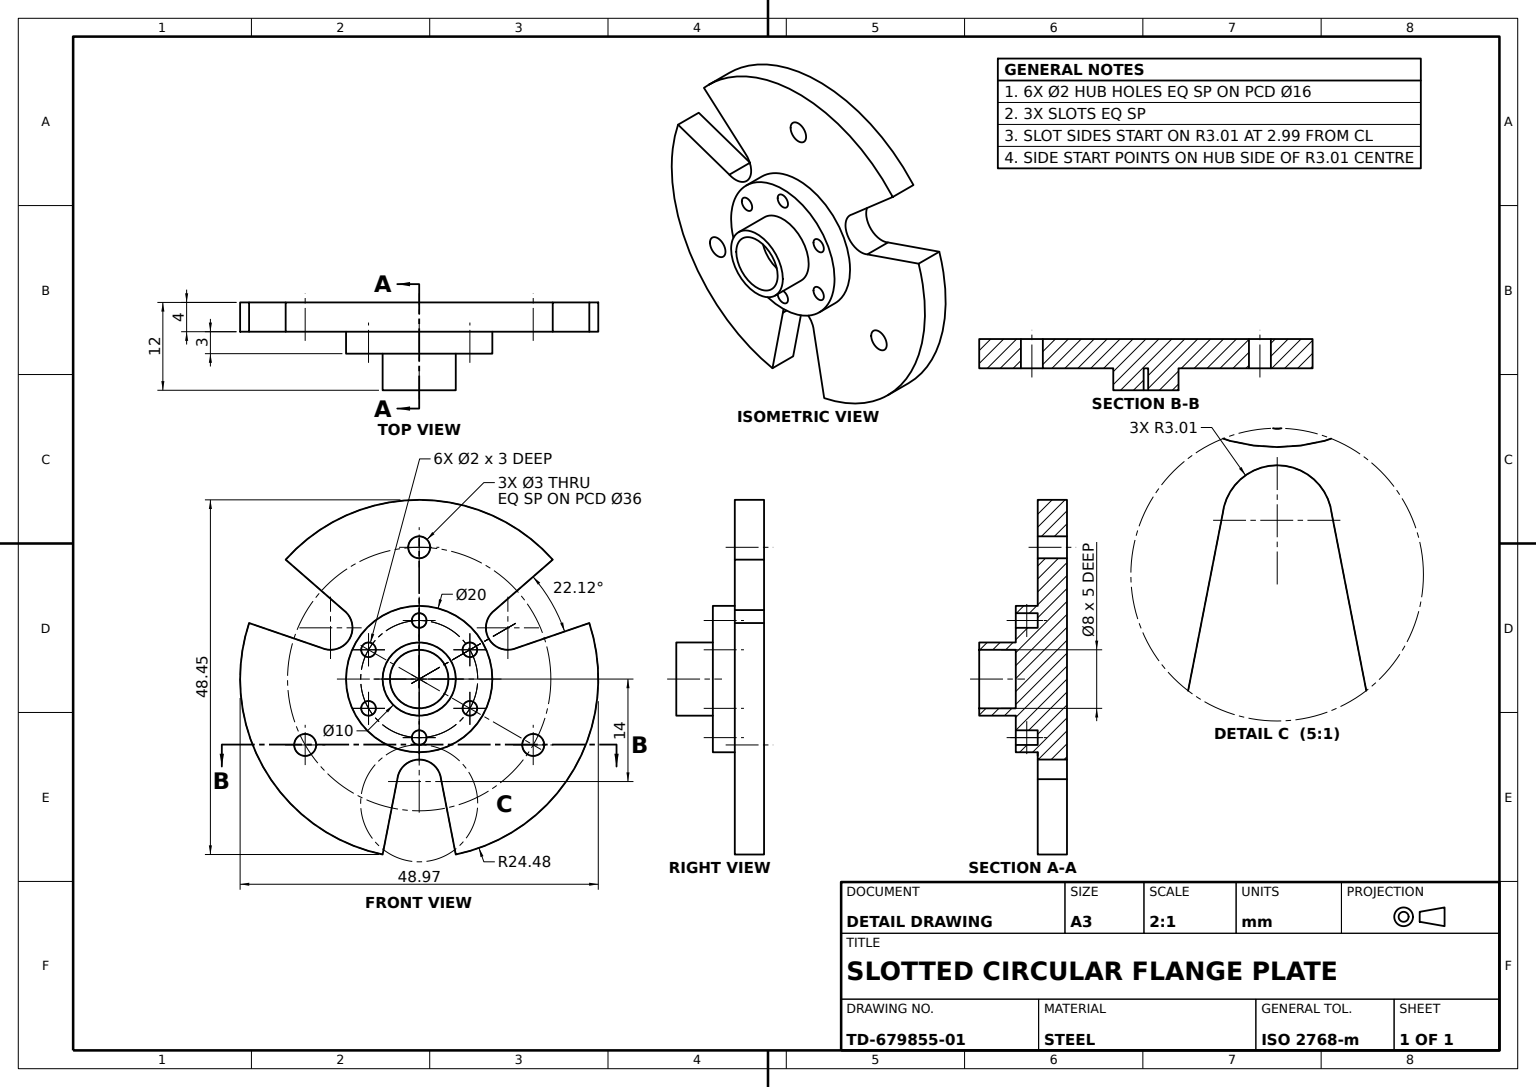
from build123d import *

# Parameters (mm, degrees)
FLANGE_PLATE_4MM_DEPTH   = 4
OUTER_HOLES_SKETCH_R     = 1.5
OUTER_HOLES_3X_DEPTH     = 35.855955648
HUB_SKETCH_R             = 10
RAISED_HUB_DEPTH         = 7
HUB_HOLES_SKETCH_R       = 1
HUB_HOLES_6X_DEPTH       = 3
CENTRE_SLEEVE_SKETCH_R   = 5
CENTRE_SLEEVE_SKETCH_R_2 = 4
CENTRE_SLEEVE_DEPTH      = 5


with BuildPart() as part:
    # Flange Plate Sketch → Flange Plate 4mm (new body)
    with BuildSketch(Plane.XY):
        with BuildLine():
            Line((-2.988714381, -13.67726531), (-5, -23.968079232))
            ThreePointArc((-5, -23.968079232), (-21.203811369, -12.242026202), (-23.256965495, 7.653912597))
            Line((-23.256965495, 7.653912597), (-13.339216403, 4.250330076))
            ThreePointArc((-13.339216403, 4.250330076), (-9.521006176, 5.496955479), (-10.350502022, 9.426935234))
            Line((-10.350502022, 9.426935234), (-18.256965495, 16.314166635))
            ThreePointArc((-18.256965495, 16.314166635), (0, 24.484052403), (18.256965495, 16.314166635))
            Line((18.256965495, 16.314166635), (10.350502022, 9.426935234))
            ThreePointArc((10.350502022, 9.426935234), (9.521006176, 5.496955479), (13.339216403, 4.250330076))
            Line((13.339216403, 4.250330076), (23.256965495, 7.653912597))
            ThreePointArc((23.256965495, 7.653912597), (21.203811369, -12.242026202), (5, -23.968079232))
            Line((5, -23.968079232), (2.988714381, -13.67726531))
            ThreePointArc((2.988714381, -13.67726531), (0, -10.993910957), (-2.988714381, -13.67726531))
        make_face()
    extrude(amount=FLANGE_PLATE_4MM_DEPTH)

    # Outer Holes Sketch → Outer Holes 3x (cut, through all)
    with BuildSketch(Plane.XY):
        with Locations((0, 18)):
            Circle(OUTER_HOLES_SKETCH_R)
        with Locations((15.588457268, -9)):
            Circle(OUTER_HOLES_SKETCH_R)
        with Locations((-15.588457268, -9)):
            Circle(OUTER_HOLES_SKETCH_R)
    extrude(amount=OUTER_HOLES_3X_DEPTH, mode=Mode.SUBTRACT)

    # Hub Sketch → Raised Hub (add)
    with BuildSketch(Plane.XY):
        Circle(HUB_SKETCH_R)
    extrude(amount=RAISED_HUB_DEPTH)

    # Hub Holes Sketch → Hub Holes 6x (cut)
    with BuildSketch(Plane.XY.offset(7)):
        with Locations((0, 8)):
            Circle(HUB_HOLES_SKETCH_R)
        with Locations((6.92870323, 4.000866025)):
            Circle(HUB_HOLES_SKETCH_R)
        with Locations((6.92970323, -3.999133975)):
            Circle(HUB_HOLES_SKETCH_R)
        with Locations((0.002, -8)):
            Circle(HUB_HOLES_SKETCH_R)
        with Locations((-6.92670323, -4.000866025)):
            Circle(HUB_HOLES_SKETCH_R)
        with Locations((-6.92770323, 3.999133975)):
            Circle(HUB_HOLES_SKETCH_R)
    extrude(amount=-HUB_HOLES_6X_DEPTH, mode=Mode.SUBTRACT)

    # Centre Sleeve Sketch → Centre Sleeve (add)
    with BuildSketch(Plane.XY.offset(7)):
        Circle(CENTRE_SLEEVE_SKETCH_R)
        Circle(CENTRE_SLEEVE_SKETCH_R_2, mode=Mode.SUBTRACT)
    extrude(amount=CENTRE_SLEEVE_DEPTH)


solid = part.part
